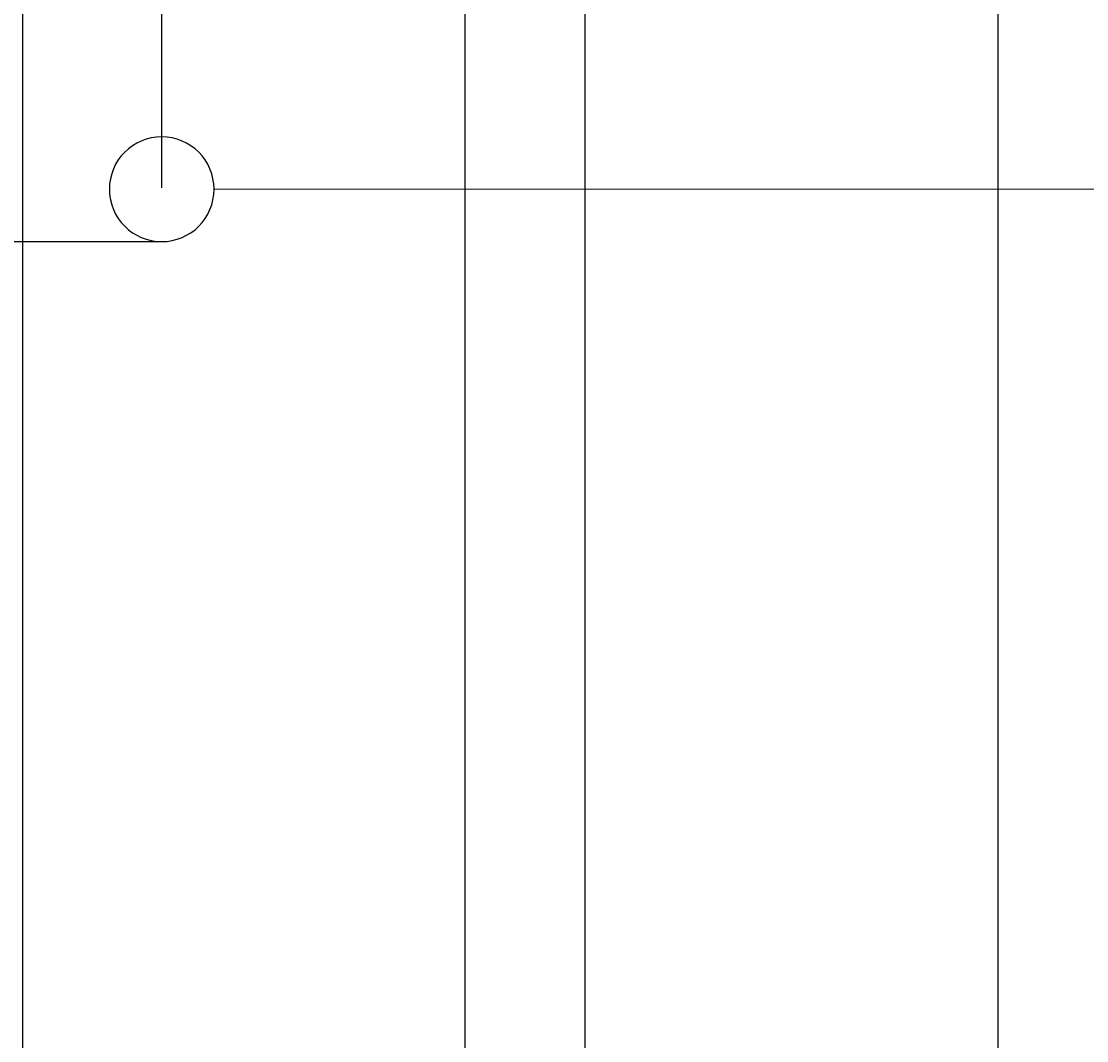
# Model space of a CAD drawing. Units: inches. Extents: x 738 to 1068, y 378 to 757.
# Tile 35 of 41: x 809 to 860, y 606 to 655. Entities that reach past the tile are written whole.
import ezdxf

# ---------------------------------------------------------------- set-up
doc = ezdxf.new("R2010")
doc.units = ezdxf.units.IN
doc.header["$MEASUREMENT"] = 0
for name, color, linetype, lineweight in [('A-ANNO-DIMS', 2, 'Continuous', 18), ('E-CTRL-PBTN', 4, 'Continuous', 25), ('E-CTRL-WIRE', 7, 'Continuous', 18)]:
    doc.layers.add(name, color=color, linetype=linetype, lineweight=lineweight)
doc.styles.get("Standard").update_dxf_attribs({"font": 'arial.ttf'})
doc.dimstyles.get("Standard").update_dxf_attribs({"dimtxt": 0.18, "dimasz": 0.18, "dimexe": 0.18, "dimexo": 0.0625, "dimgap": 0.09, "dimtad": 0, "dimtih": 1, "dimtoh": 1, "dimdec": 4, "dimzin": 0, "dimdsep": 46, "dimtxsty": 'Standard', "dimcen": 0.09, "dimadec": 0, "dimazin": 0, "dimtfac": 1, "dimtdec": 4, "dimtofl": 0, "dimtmove": 0, "dimatfit": 3, "dimfxl": 1, "dimtolj": 1, "dimtzin": 0, "dimarcsym": 0})

# ---------------------------------------------------------------- blocks, each defined once
blk = doc.blocks.new('*D26')
at = {"layer": 'A-ANNO-DIMS', "color": 0, "lineweight": -2, "transparency": 16777216}
for p, q in [((816.008, 647.048), (816.008, 756.505)), ((867.596, 647.048), (867.596, 756.505)), ((816.188, 756.325), (841.408, 756.325)), ((867.416, 756.325), (842.196, 756.325))]:
    blk.add_line(p, q, dxfattribs=at)
at = {"layer": 'A-ANNO-DIMS', "color": 0, "transparency": 16777216}
for points in [[(816.188, 756.355), (816.188, 756.295), (816.008, 756.325)], [(867.416, 756.355), (867.416, 756.295), (867.596, 756.325)]]:
    blk.add_solid(points, dxfattribs=at)
at = {"layer": 'Defpoints', "color": 0, "transparency": 16777216}
for p in [(867.596, 756.325), (816.008, 646.985), (867.596, 646.985)]:
    blk.add_point(p, dxfattribs=at)
at = {"layer": 'A-ANNO-DIMS', "color": 0, "transparency": 16777216, "insert": (841.802, 756.325), "char_height": 0.18, "attachment_point": 5}
blk.add_mtext('\\A1;51.59', dxfattribs=at)
blk = doc.blocks.new('*D32')
at = {"layer": 'A-ANNO-DIMS', "color": 0, "lineweight": -2, "transparency": 16777216}
for p, q in [((809.38, 461.454), (809.38, 756.505)), ((836.232, 461.277), (836.232, 756.505)), ((809.56, 756.325), (822.41, 756.325)), ((836.052, 756.325), (823.202, 756.325))]:
    blk.add_line(p, q, dxfattribs=at)
at = {"layer": 'A-ANNO-DIMS', "color": 0, "transparency": 16777216}
for points in [[(809.56, 756.355), (809.56, 756.295), (809.38, 756.325)], [(836.052, 756.355), (836.052, 756.295), (836.232, 756.325)]]:
    blk.add_solid(points, dxfattribs=at)
at = {"layer": 'Defpoints', "color": 0, "transparency": 16777216}
for p in [(836.232, 756.325), (809.38, 461.392), (836.232, 461.214)]:
    blk.add_point(p, dxfattribs=at)
at = {"layer": 'A-ANNO-DIMS', "color": 0, "transparency": 16777216, "insert": (822.806, 756.325), "char_height": 0.18, "attachment_point": 5}
blk.add_mtext('\\A1;26.85', dxfattribs=at)
blk = doc.blocks.new('*D34')
at = {"layer": 'A-ANNO-DIMS', "color": 0, "lineweight": -2, "transparency": 16777216}
for p, q in [((781.49, 686.266), (781.49, 378.239)), ((830.489, 686.266), (830.489, 378.239)), ((781.67, 378.419), (805.767, 378.419)), ((830.309, 378.419), (806.212, 378.419))]:
    blk.add_line(p, q, dxfattribs=at)
at = {"layer": 'A-ANNO-DIMS', "color": 0, "transparency": 16777216}
for points in [[(781.67, 378.449), (781.67, 378.389), (781.49, 378.419)], [(830.309, 378.449), (830.309, 378.389), (830.489, 378.419)]]:
    blk.add_solid(points, dxfattribs=at)
at = {"layer": 'Defpoints', "color": 0, "transparency": 16777216}
for p in [(781.49, 686.329), (830.489, 686.329), (830.489, 378.419)]:
    blk.add_point(p, dxfattribs=at)
at = {"layer": 'A-ANNO-DIMS', "color": 0, "transparency": 16777216, "insert": (805.99, 378.419), "char_height": 0.18, "attachment_point": 5}
blk.add_mtext('\\A1;49', dxfattribs=at)
blk = doc.blocks.new('*D35')
at = {"layer": 'A-ANNO-DIMS', "color": 0, "lineweight": -2, "transparency": 16777216}
for p, q in [((855.932, 686.266), (855.932, 378.239)), ((901.429, 686.267), (901.429, 378.239)), ((856.112, 378.419), (878.352, 378.419)), ((901.249, 378.419), (879.009, 378.419))]:
    blk.add_line(p, q, dxfattribs=at)
at = {"layer": 'A-ANNO-DIMS', "color": 0, "transparency": 16777216}
for points in [[(856.112, 378.449), (856.112, 378.389), (855.932, 378.419)], [(901.249, 378.449), (901.249, 378.389), (901.429, 378.419)]]:
    blk.add_solid(points, dxfattribs=at)
at = {"layer": 'Defpoints', "color": 0, "transparency": 16777216}
for p in [(855.932, 686.329), (901.429, 686.329), (901.429, 378.419)]:
    blk.add_point(p, dxfattribs=at)
at = {"layer": 'A-ANNO-DIMS', "color": 0, "transparency": 16777216, "insert": (878.68, 378.419), "char_height": 0.18, "attachment_point": 5}
blk.add_mtext('\\A1;45.5', dxfattribs=at)

msp = doc.modelspace()

# ---------------------------------------------------------------- linework, layer by layer
at = {"layer": 'E-CTRL-PBTN'}
msp.add_line((803.5218, 644.4853), (816.0076, 644.4853), dxfattribs=at)
msp.add_lwpolyline([(813.5076, 646.9853, 1), (818.5076, 646.9853, 1)], format="xyb", close=True, dxfattribs=at)
at = {"layer": 'E-CTRL-WIRE'}
msp.add_line((818.5076, 646.9853), (865.0964, 646.9853), dxfattribs=at)

# ---------------------------------------------------------------- dimensions: what is measured, and where the dimension line sits
at = {"layer": 'A-ANNO-DIMS'}
for base, p1, p2, override, picture, middle in [((836.2324, 756.3251), (809.3803, 461.3919), (836.2324, 461.214), {"dimdec": 2, "dimlfac": 1, "dimrnd": 0, "dimzin": 0, "dimdsep": 46, "dimlunit": 2}, '*D32', (822.8064, 756.3251)), ((867.5964, 756.3251), (816.0076, 646.9853), (867.5964, 646.9853), {"dimdec": 2, "dimlfac": 1, "dimrnd": 0, "dimzin": 0, "dimdsep": 46, "dimlunit": 2}, '*D26', (841.802, 756.3251)), ((830.4893, 378.4191), (781.4897, 686.329), (830.4893, 686.329), {"dimdec": 0, "dimlfac": 1, "dimrnd": 0, "dimzin": 0, "dimdsep": 46, "dimlunit": 2}, '*D34', (805.9895, 378.4191)), ((901.4286, 378.4191), (855.9323, 686.329), (901.4286, 686.3292), {"dimdec": 1, "dimlfac": 1, "dimrnd": 0, "dimzin": 0, "dimdsep": 46, "dimlunit": 2}, '*D35', (878.6804, 378.4191))]:
    dim = msp.add_linear_dim(base=base, p1=p1, p2=p2, dimstyle='Standard', override=override, dxfattribs=at)
    dim.commit()
    dim.dimension.update_dxf_attribs({"geometry": picture, "text_midpoint": middle})

doc.saveas('drawing.dxf')
